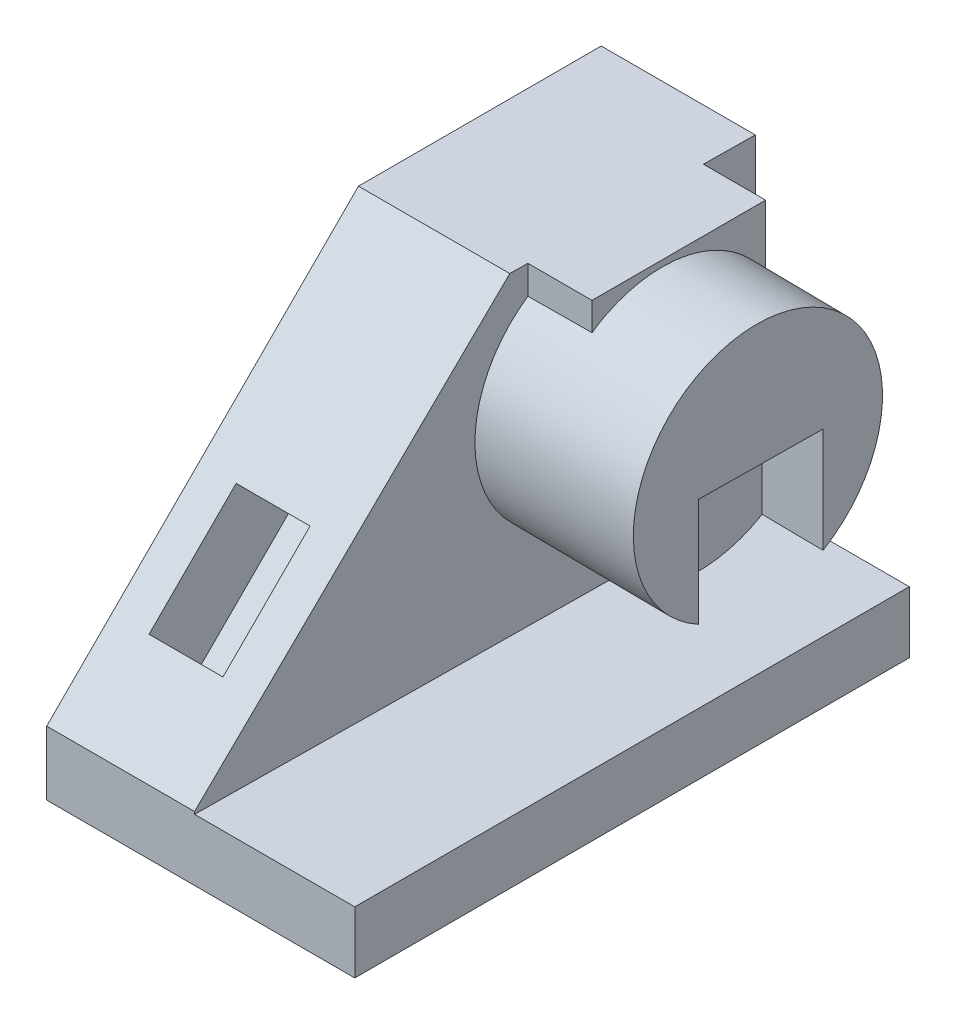
ISO-10303-21;
HEADER;
FILE_DESCRIPTION(('STEP AP214'),'2;1');
FILE_NAME('part.step','',(''),(''),'','','');
FILE_SCHEMA(('AUTOMOTIVE_DESIGN { 1 0 10303 214 1 1 1 1 }'));
ENDSEC;
DATA;
#1=APPLICATION_CONTEXT('core data for automotive mechanical design processes');
#2=APPLICATION_PROTOCOL_DEFINITION('international standard','automotive_design',2000,#1);
#3=PRODUCT_CONTEXT('',#1,'mechanical');
#4=PRODUCT('Part','Part','',(#3));
#5=PRODUCT_RELATED_PRODUCT_CATEGORY('part','',(#4));
#6=PRODUCT_DEFINITION_FORMATION('','',#4);
#7=PRODUCT_DEFINITION_CONTEXT('part definition',#1,'design');
#8=PRODUCT_DEFINITION('design','',#6,#7);
#9=PRODUCT_DEFINITION_SHAPE('','',#8);
#10=(LENGTH_UNIT() NAMED_UNIT(*) SI_UNIT(.MILLI.,.METRE.));
#11=(NAMED_UNIT(*) PLANE_ANGLE_UNIT() SI_UNIT($,.RADIAN.));
#12=(NAMED_UNIT(*) SI_UNIT($,.STERADIAN.) SOLID_ANGLE_UNIT());
#13=UNCERTAINTY_MEASURE_WITH_UNIT(LENGTH_MEASURE(1.E-05),#10,'distance_accuracy_value','');
#14=(GEOMETRIC_REPRESENTATION_CONTEXT(3) GLOBAL_UNCERTAINTY_ASSIGNED_CONTEXT((#13)) GLOBAL_UNIT_ASSIGNED_CONTEXT((#10,
#11,#12)) REPRESENTATION_CONTEXT('',''));
#15=CARTESIAN_POINT('',(0.,0.,0.));
#16=DIRECTION('',(0.,0.,1.));
#17=DIRECTION('',(1.,0.,0.));
#18=AXIS2_PLACEMENT_3D('',#15,#16,#17);
#19=CARTESIAN_POINT('',(-15.4419889502762,10.,45.));
#20=DIRECTION('',(1.,0.,0.));
#21=DIRECTION('',(0.,0.,-1.));
#22=AXIS2_PLACEMENT_3D('',#19,#20,#21);
#23=PLANE('',#22);
#24=DIRECTION('',(0.,-1.,0.));
#25=VECTOR('',#24,1.);
#26=CARTESIAN_POINT('',(-15.4419889502762,10.,45.));
#27=LINE('',#26,#25);
#28=CARTESIAN_POINT('',(-15.4419889502763,10.4020202535532,45.));
#29=VERTEX_POINT('',#28);
#30=CARTESIAN_POINT('',(-15.4419889502762,0.,45.));
#31=VERTEX_POINT('',#30);
#32=EDGE_CURVE('E303',#29,#31,#27,.T.);
#33=ORIENTED_EDGE('',*,*,#32,.F.);
#34=DIRECTION('',(0.,-0.707106781186549,0.707106781186546));
#35=VECTOR('',#34,1.);
#36=CARTESIAN_POINT('',(-15.4419889502763,-28.4088608780224,83.8108811315755));
#37=LINE('',#36,#35);
#38=CARTESIAN_POINT('',(-15.4419889502762,61.,-5.59797974644655));
#39=VERTEX_POINT('',#38);
#40=EDGE_CURVE('E203',#39,#29,#37,.T.);
#41=ORIENTED_EDGE('',*,*,#40,.F.);
#42=DIRECTION('',(0.,0.,1.));
#43=VECTOR('',#42,1.);
#44=CARTESIAN_POINT('',(-15.4419889502763,61.,-45.));
#45=LINE('',#44,#43);
#46=CARTESIAN_POINT('',(-15.4419889502763,61.,-45.));
#47=VERTEX_POINT('',#46);
#48=EDGE_CURVE('E220',#47,#39,#45,.T.);
#49=ORIENTED_EDGE('',*,*,#48,.F.);
#50=DIRECTION('',(0.,-1.,0.));
#51=VECTOR('',#50,1.);
#52=CARTESIAN_POINT('',(-15.4419889502762,10.,-45.));
#53=LINE('',#52,#51);
#54=CARTESIAN_POINT('',(-15.4419889502762,0.,-45.));
#55=VERTEX_POINT('',#54);
#56=EDGE_CURVE('E290',#47,#55,#53,.T.);
#57=ORIENTED_EDGE('',*,*,#56,.T.);
#58=DIRECTION('',(0.,0.,1.));
#59=VECTOR('',#58,1.);
#60=CARTESIAN_POINT('',(-15.4419889502762,0.,45.));
#61=LINE('',#60,#59);
#62=EDGE_CURVE('E280',#55,#31,#61,.T.);
#63=ORIENTED_EDGE('',*,*,#62,.T.);
#64=EDGE_LOOP('',(#33,#41,#49,#57,#63));
#65=FACE_BOUND('',#64,.T.);
#66=ADVANCED_FACE('F41',(#65),#23,.F.);
#67=CARTESIAN_POINT('',(34.5580110497238,10.,45.));
#68=DIRECTION('',(0.,0.,-1.));
#69=DIRECTION('',(-1.,0.,0.));
#70=AXIS2_PLACEMENT_3D('',#67,#68,#69);
#71=PLANE('',#70);
#72=DIRECTION('',(0.,-1.,0.));
#73=VECTOR('',#72,1.);
#74=CARTESIAN_POINT('',(8.55801104972375,60.,45.));
#75=LINE('',#74,#73);
#76=CARTESIAN_POINT('',(8.55801104972375,10.4020202535532,45.));
#77=VERTEX_POINT('',#76);
#78=CARTESIAN_POINT('',(8.55801104972376,10.,45.));
#79=VERTEX_POINT('',#78);
#80=EDGE_CURVE('E279',#77,#79,#75,.T.);
#81=ORIENTED_EDGE('',*,*,#80,.F.);
#82=DIRECTION('',(-1.,0.,0.));
#83=VECTOR('',#82,1.);
#84=CARTESIAN_POINT('',(34.5580110497238,10.4020202535532,45.));
#85=LINE('',#84,#83);
#86=EDGE_CURVE('E214',#77,#29,#85,.T.);
#87=ORIENTED_EDGE('',*,*,#86,.T.);
#88=ORIENTED_EDGE('',*,*,#32,.T.);
#89=DIRECTION('',(1.,0.,0.));
#90=VECTOR('',#89,1.);
#91=CARTESIAN_POINT('',(34.5580110497238,0.,45.));
#92=LINE('',#91,#90);
#93=CARTESIAN_POINT('',(34.5580110497238,0.,45.));
#94=VERTEX_POINT('',#93);
#95=EDGE_CURVE('E288',#31,#94,#92,.T.);
#96=ORIENTED_EDGE('',*,*,#95,.T.);
#97=DIRECTION('',(0.,-1.,0.));
#98=VECTOR('',#97,1.);
#99=CARTESIAN_POINT('',(34.5580110497238,10.,45.));
#100=LINE('',#99,#98);
#101=CARTESIAN_POINT('',(34.5580110497238,10.,45.));
#102=VERTEX_POINT('',#101);
#103=EDGE_CURVE('E297',#102,#94,#100,.T.);
#104=ORIENTED_EDGE('',*,*,#103,.F.);
#105=DIRECTION('',(1.,0.,0.));
#106=VECTOR('',#105,1.);
#107=CARTESIAN_POINT('',(34.5580110497238,10.,45.));
#108=LINE('',#107,#106);
#109=EDGE_CURVE('E278',#79,#102,#108,.T.);
#110=ORIENTED_EDGE('',*,*,#109,.F.);
#111=EDGE_LOOP('',(#81,#87,#88,#96,#104,#110));
#112=FACE_BOUND('',#111,.T.);
#113=ADVANCED_FACE('F360',(#112),#71,.F.);
#114=CARTESIAN_POINT('',(34.5580110497238,10.,45.));
#115=DIRECTION('',(-1.,0.,0.));
#116=DIRECTION('',(0.,0.,1.));
#117=AXIS2_PLACEMENT_3D('',#114,#115,#116);
#118=PLANE('',#117);
#119=DIRECTION('',(0.,0.,-1.));
#120=VECTOR('',#119,1.);
#121=CARTESIAN_POINT('',(34.5580110497238,0.,45.));
#122=LINE('',#121,#120);
#123=CARTESIAN_POINT('',(34.5580110497238,0.,-45.));
#124=VERTEX_POINT('',#123);
#125=EDGE_CURVE('E292',#94,#124,#122,.T.);
#126=ORIENTED_EDGE('',*,*,#125,.T.);
#127=DIRECTION('',(0.,-1.,0.));
#128=VECTOR('',#127,1.);
#129=CARTESIAN_POINT('',(34.5580110497238,10.,-45.));
#130=LINE('',#129,#128);
#131=CARTESIAN_POINT('',(34.5580110497238,10.,-45.));
#132=VERTEX_POINT('',#131);
#133=EDGE_CURVE('E300',#132,#124,#130,.T.);
#134=ORIENTED_EDGE('',*,*,#133,.F.);
#135=DIRECTION('',(0.,0.,-1.));
#136=VECTOR('',#135,1.);
#137=CARTESIAN_POINT('',(34.5580110497238,10.,45.));
#138=LINE('',#137,#136);
#139=EDGE_CURVE('E281',#102,#132,#138,.T.);
#140=ORIENTED_EDGE('',*,*,#139,.F.);
#141=ORIENTED_EDGE('',*,*,#103,.T.);
#142=EDGE_LOOP('',(#126,#134,#140,#141));
#143=FACE_BOUND('',#142,.T.);
#144=ADVANCED_FACE('F361',(#143),#118,.F.);
#145=CARTESIAN_POINT('',(34.5580110497238,10.,-45.));
#146=DIRECTION('',(0.,0.,1.));
#147=DIRECTION('',(1.,0.,0.));
#148=AXIS2_PLACEMENT_3D('',#145,#146,#147);
#149=PLANE('',#148);
#150=DIRECTION('',(0.,-1.,0.));
#151=VECTOR('',#150,1.);
#152=CARTESIAN_POINT('',(9.55801104972376,60.,-45.));
#153=LINE('',#152,#151);
#154=CARTESIAN_POINT('',(9.55801104972376,61.,-45.));
#155=VERTEX_POINT('',#154);
#156=CARTESIAN_POINT('',(9.55801104972376,10.,-45.));
#157=VERTEX_POINT('',#156);
#158=EDGE_CURVE('E274',#155,#157,#153,.T.);
#159=ORIENTED_EDGE('',*,*,#158,.T.);
#160=DIRECTION('',(-1.,0.,0.));
#161=VECTOR('',#160,1.);
#162=CARTESIAN_POINT('',(34.5580110497238,10.,-45.));
#163=LINE('',#162,#161);
#164=EDGE_CURVE('E282',#132,#157,#163,.T.);
#165=ORIENTED_EDGE('',*,*,#164,.F.);
#166=ORIENTED_EDGE('',*,*,#133,.T.);
#167=DIRECTION('',(-1.,0.,0.));
#168=VECTOR('',#167,1.);
#169=CARTESIAN_POINT('',(34.5580110497238,0.,-45.));
#170=LINE('',#169,#168);
#171=EDGE_CURVE('E285',#124,#55,#170,.T.);
#172=ORIENTED_EDGE('',*,*,#171,.T.);
#173=ORIENTED_EDGE('',*,*,#56,.F.);
#174=DIRECTION('',(-1.,0.,0.));
#175=VECTOR('',#174,1.);
#176=CARTESIAN_POINT('',(9.55801104972376,61.,-45.));
#177=LINE('',#176,#175);
#178=EDGE_CURVE('E213',#155,#47,#177,.T.);
#179=ORIENTED_EDGE('',*,*,#178,.F.);
#180=EDGE_LOOP('',(#159,#165,#166,#172,#173,#179));
#181=FACE_BOUND('',#180,.T.);
#182=ADVANCED_FACE('F331',(#181),#149,.F.);
#183=CARTESIAN_POINT('',(0.,10.,0.));
#184=DIRECTION('',(0.,1.,0.));
#185=DIRECTION('',(0.,0.,1.));
#186=AXIS2_PLACEMENT_3D('',#183,#184,#185);
#187=PLANE('',#186);
#188=DIRECTION('',(0.011110425303555,0.,-0.999938277319943));
#189=VECTOR('',#188,1.);
#190=CARTESIAN_POINT('',(8.55801104972375,10.,45.));
#191=LINE('',#190,#189);
#192=EDGE_CURVE('E268',#79,#157,#191,.T.);
#193=ORIENTED_EDGE('',*,*,#192,.F.);
#194=ORIENTED_EDGE('',*,*,#109,.T.);
#195=ORIENTED_EDGE('',*,*,#139,.T.);
#196=ORIENTED_EDGE('',*,*,#164,.T.);
#197=EDGE_LOOP('',(#193,#194,#195,#196));
#198=FACE_BOUND('',#197,.T.);
#199=ADVANCED_FACE('F372',(#198),#187,.T.);
#200=CARTESIAN_POINT('',(0.,0.,0.));
#201=DIRECTION('',(0.,1.,0.));
#202=DIRECTION('',(0.,0.,1.));
#203=AXIS2_PLACEMENT_3D('',#200,#201,#202);
#204=PLANE('',#203);
#205=ORIENTED_EDGE('',*,*,#62,.F.);
#206=ORIENTED_EDGE('',*,*,#171,.F.);
#207=ORIENTED_EDGE('',*,*,#125,.F.);
#208=ORIENTED_EDGE('',*,*,#95,.F.);
#209=EDGE_LOOP('',(#205,#206,#207,#208));
#210=FACE_BOUND('',#209,.T.);
#211=ADVANCED_FACE('F374',(#210),#204,.F.);
#212=CARTESIAN_POINT('',(8.55801104972375,60.,45.));
#213=DIRECTION('',(-0.999938277319942,0.,-0.011110425303555));
#214=DIRECTION('',(-0.011110425303555,0.,0.999938277319942));
#215=AXIS2_PLACEMENT_3D('',#212,#213,#214);
#216=PLANE('',#215);
#217=DIRECTION('',(0.0111104253035549,0.,-0.999938277319942));
#218=VECTOR('',#217,1.);
#219=CARTESIAN_POINT('',(9.0024554941682,61.,5.));
#220=LINE('',#219,#218);
#221=CARTESIAN_POINT('',(9.12021082468428,61.,-5.59797974644659));
#222=VERTEX_POINT('',#221);
#223=CARTESIAN_POINT('',(9.15254596288799,61.,-8.50814218478106));
#224=VERTEX_POINT('',#223);
#225=EDGE_CURVE('E219',#222,#224,#220,.T.);
#226=ORIENTED_EDGE('',*,*,#225,.F.);
#227=DIRECTION('',(-0.00785649953237235,-0.70708495791351,0.707084957913508));
#228=VECTOR('',#227,1.);
#229=CARTESIAN_POINT('',(8.83353837378895,35.1994794194208,20.2025408341325));
#230=LINE('',#229,#228);
#231=EDGE_CURVE('E61',#222,#77,#230,.T.);
#232=ORIENTED_EDGE('',*,*,#231,.T.);
#233=ORIENTED_EDGE('',*,*,#80,.T.);
#234=ORIENTED_EDGE('',*,*,#192,.T.);
#235=ORIENTED_EDGE('',*,*,#158,.F.);
#236=DIRECTION('',(0.0111104253035545,0.,-0.999938277319942));
#237=VECTOR('',#236,1.);
#238=CARTESIAN_POINT('',(9.46553831809246,61.,-36.6774541531825));
#239=LINE('',#238,#237);
#240=CARTESIAN_POINT('',(9.46553831809246,61.,-36.6774541531825));
#241=VERTEX_POINT('',#240);
#242=EDGE_CURVE('E233',#241,#155,#239,.T.);
#243=ORIENTED_EDGE('',*,*,#242,.F.);
#244=DIRECTION('',(0.,1.,0.));
#245=VECTOR('',#244,1.);
#246=CARTESIAN_POINT('',(9.46553831809246,40.,-36.6774541531825));
#247=LINE('',#246,#245);
#248=CARTESIAN_POINT('',(9.46553831809246,51.039912039484,-36.6774541531825));
#249=VERTEX_POINT('',#248);
#250=EDGE_CURVE('E232',#249,#241,#247,.T.);
#251=ORIENTED_EDGE('',*,*,#250,.F.);
#252=CARTESIAN_POINT('',(9.28025041713489,40.,-20.0015430670015));
#253=DIRECTION('',(0.999938277319943,0.,0.011110425303555));
#254=DIRECTION('',(0.011110425303555,0.,-0.999938277319943));
#255=AXIS2_PLACEMENT_3D('',#252,#253,#254);
#256=CIRCLE('',#255,20.);
#257=CARTESIAN_POINT('',(9.15254596288799,56.3672058621177,-8.50814218478106));
#258=VERTEX_POINT('',#257);
#259=EDGE_CURVE('E267',#258,#249,#256,.T.);
#260=ORIENTED_EDGE('',*,*,#259,.F.);
#261=DIRECTION('',(0.,1.,0.));
#262=VECTOR('',#261,1.);
#263=CARTESIAN_POINT('',(9.15254596288799,40.,-8.50814218478106));
#264=LINE('',#263,#262);
#265=EDGE_CURVE('E234',#258,#224,#264,.T.);
#266=ORIENTED_EDGE('',*,*,#265,.T.);
#267=EDGE_LOOP('',(#226,#232,#233,#234,#235,#243,#251,#260,#266));
#268=FACE_BOUND('',#267,.T.);
#269=ADVANCED_FACE('F328',(#268),#216,.F.);
#270=CARTESIAN_POINT('',(35.2786456274534,40.,-19.712672009109));
#271=DIRECTION('',(-0.999938277319943,0.,-0.011110425303555));
#272=DIRECTION('',(-0.011110425303555,0.,0.999938277319943));
#273=AXIS2_PLACEMENT_3D('',#270,#271,#272);
#274=CYLINDRICAL_SURFACE('',#273,20.);
#275=CARTESIAN_POINT('',(35.2786456274534,40.,-19.712672009109));
#276=DIRECTION('',(0.999938277319943,0.,0.011110425303555));
#277=DIRECTION('',(0.011110425303555,0.,-0.999938277319943));
#278=AXIS2_PLACEMENT_3D('',#275,#276,#277);
#279=CIRCLE('',#278,20.);
#280=CARTESIAN_POINT('',(35.3948087110377,22.9504773076578,-30.1673495316977));
#281=VERTEX_POINT('',#280);
#282=CARTESIAN_POINT('',(35.1726002049666,22.4244733176461,-10.1685839852988));
#283=VERTEX_POINT('',#282);
#284=EDGE_CURVE('E270',#281,#283,#279,.T.);
#285=ORIENTED_EDGE('',*,*,#284,.F.);
#286=DIRECTION('',(-0.999938277319943,0.,-0.011110425303555));
#287=VECTOR('',#286,1.);
#288=CARTESIAN_POINT('',(35.3948087110377,22.9504773076578,-30.1673495316977));
#289=LINE('',#288,#287);
#290=CARTESIAN_POINT('',(25.3954259378383,22.9504773076578,-30.2784537847332));
#291=VERTEX_POINT('',#290);
#292=EDGE_CURVE('E263',#281,#291,#289,.T.);
#293=ORIENTED_EDGE('',*,*,#292,.T.);
#294=CARTESIAN_POINT('',(25.279262854254,40.,-19.8237762621446));
#295=DIRECTION('',(0.999938277319943,0.,0.011110425303555));
#296=DIRECTION('',(0.011110425303555,0.,-0.999938277319943));
#297=AXIS2_PLACEMENT_3D('',#294,#295,#296);
#298=CIRCLE('',#297,20.);
#299=CARTESIAN_POINT('',(25.1732174317672,22.4244733176461,-10.2796882383344));
#300=VERTEX_POINT('',#299);
#301=EDGE_CURVE('E308',#300,#291,#298,.T.);
#302=ORIENTED_EDGE('',*,*,#301,.F.);
#303=DIRECTION('',(-0.999938277319943,0.,-0.011110425303555));
#304=VECTOR('',#303,1.);
#305=CARTESIAN_POINT('',(35.1726002049666,22.4244733176461,-10.1685839852988));
#306=LINE('',#305,#304);
#307=EDGE_CURVE('E258',#300,#283,#306,.F.);
#308=ORIENTED_EDGE('',*,*,#307,.T.);
#309=EDGE_LOOP('',(#285,#293,#302,#308));
#310=FACE_BOUND('',#309,.T.);
#311=ORIENTED_EDGE('',*,*,#259,.T.);
#312=CARTESIAN_POINT('',(-1491.55174733915,40.,-36.6774541531825));
#313=DIRECTION('',(0.,0.,-1.));
#314=DIRECTION('',(-1.,0.,0.));
#315=AXIS2_PLACEMENT_3D('',#312,#313,#314);
#316=ELLIPSE('',#315,1800.11110768196,20.);
#317=CARTESIAN_POINT('',(19.5580110497238,50.8686272432883,-36.6774541531825));
#318=VERTEX_POINT('',#317);
#319=EDGE_CURVE('E48',#249,#318,#316,.T.);
#320=ORIENTED_EDGE('',*,*,#319,.T.);
#321=CARTESIAN_POINT('',(19.5580110497238,40.,-19.8873457266394));
#322=DIRECTION('',(1.,0.,0.));
#323=DIRECTION('',(0.,0.,-1.));
#324=AXIS2_PLACEMENT_3D('',#321,#322,#323);
#325=ELLIPSE('',#324,20.0012345297996,20.);
#326=CARTESIAN_POINT('',(19.5580110497238,56.4477874116639,-8.50814218478106));
#327=VERTEX_POINT('',#326);
#328=EDGE_CURVE('E312',#318,#327,#325,.T.);
#329=ORIENTED_EDGE('',*,*,#328,.T.);
#330=CARTESIAN_POINT('',(1043.68632981697,40.,-8.50814218478106));
#331=DIRECTION('',(0.,0.,1.));
#332=DIRECTION('',(-1.,0.,0.));
#333=AXIS2_PLACEMENT_3D('',#330,#331,#332);
#334=ELLIPSE('',#333,1800.11110768196,20.);
#335=EDGE_CURVE('E309',#327,#258,#334,.T.);
#336=ORIENTED_EDGE('',*,*,#335,.T.);
#337=EDGE_LOOP('',(#311,#320,#329,#336));
#338=FACE_BOUND('',#337,.T.);
#339=ADVANCED_FACE('F319',(#310,#338),#274,.T.);
#340=CARTESIAN_POINT('',(35.2786456274534,40.,-19.712672009109));
#341=DIRECTION('',(0.999938277319943,0.,0.011110425303555));
#342=DIRECTION('',(0.011110425303555,0.,-0.999938277319943));
#343=AXIS2_PLACEMENT_3D('',#340,#341,#342);
#344=PLANE('',#343);
#345=DIRECTION('',(0.,1.,0.));
#346=VECTOR('',#345,1.);
#347=CARTESIAN_POINT('',(35.3948087110377,40.,-30.1673495316977));
#348=LINE('',#347,#346);
#349=CARTESIAN_POINT('',(35.3948087110377,40.,-30.1673495316988));
#350=VERTEX_POINT('',#349);
#351=EDGE_CURVE('E304',#281,#350,#348,.T.);
#352=ORIENTED_EDGE('',*,*,#351,.F.);
#353=ORIENTED_EDGE('',*,*,#284,.T.);
#354=DIRECTION('',(0.,-1.,0.));
#355=VECTOR('',#354,1.);
#356=CARTESIAN_POINT('',(35.1726002049666,40.,-10.1685839852988));
#357=LINE('',#356,#355);
#358=CARTESIAN_POINT('',(35.1726002049666,40.,-10.1685839852988));
#359=VERTEX_POINT('',#358);
#360=EDGE_CURVE('E250',#359,#283,#357,.T.);
#361=ORIENTED_EDGE('',*,*,#360,.F.);
#362=DIRECTION('',(-0.0111104253035552,0.,0.999938277319943));
#363=VECTOR('',#362,1.);
#364=CARTESIAN_POINT('',(35.1726002049666,40.,-10.1685839852988));
#365=LINE('',#364,#363);
#366=EDGE_CURVE('E240',#350,#359,#365,.T.);
#367=ORIENTED_EDGE('',*,*,#366,.F.);
#368=EDGE_LOOP('',(#352,#353,#361,#367));
#369=FACE_BOUND('',#368,.T.);
#370=ADVANCED_FACE('F383',(#369),#344,.T.);
#371=CARTESIAN_POINT('',(25.2843216848027,40.,-20.2790710115338));
#372=DIRECTION('',(0.999938277319943,0.,0.011110425303555));
#373=DIRECTION('',(0.011110425303555,0.,-0.999938277319943));
#374=AXIS2_PLACEMENT_3D('',#371,#372,#373);
#375=PLANE('',#374);
#376=ORIENTED_EDGE('',*,*,#301,.T.);
#377=DIRECTION('',(0.,1.,0.));
#378=VECTOR('',#377,1.);
#379=CARTESIAN_POINT('',(25.3954259378383,40.,-30.2784537847332));
#380=LINE('',#379,#378);
#381=CARTESIAN_POINT('',(25.3954259378383,40.,-30.2784537847332));
#382=VERTEX_POINT('',#381);
#383=EDGE_CURVE('E242',#291,#382,#380,.T.);
#384=ORIENTED_EDGE('',*,*,#383,.T.);
#385=DIRECTION('',(-0.0111104253035552,0.,0.999938277319943));
#386=VECTOR('',#385,1.);
#387=CARTESIAN_POINT('',(25.1732174317672,40.,-10.2796882383344));
#388=LINE('',#387,#386);
#389=CARTESIAN_POINT('',(25.1732174317672,40.,-10.2796882383344));
#390=VERTEX_POINT('',#389);
#391=EDGE_CURVE('E246',#382,#390,#388,.T.);
#392=ORIENTED_EDGE('',*,*,#391,.T.);
#393=DIRECTION('',(0.,-1.,0.));
#394=VECTOR('',#393,1.);
#395=CARTESIAN_POINT('',(25.1732174317672,40.,-10.2796882383344));
#396=LINE('',#395,#394);
#397=EDGE_CURVE('E249',#390,#300,#396,.T.);
#398=ORIENTED_EDGE('',*,*,#397,.T.);
#399=EDGE_LOOP('',(#376,#384,#392,#398));
#400=FACE_BOUND('',#399,.T.);
#401=ADVANCED_FACE('F388',(#400),#375,.T.);
#402=CARTESIAN_POINT('',(25.3954259378383,40.,-30.2784537847332));
#403=DIRECTION('',(0.011110425303555,0.,-0.999938277319943));
#404=DIRECTION('',(-0.999938277319943,0.,-0.011110425303555));
#405=AXIS2_PLACEMENT_3D('',#402,#403,#404);
#406=PLANE('',#405);
#407=ORIENTED_EDGE('',*,*,#351,.T.);
#408=DIRECTION('',(0.999938277319943,0.,0.011110425303555));
#409=VECTOR('',#408,1.);
#410=CARTESIAN_POINT('',(25.3954259378383,40.,-30.2784537847332));
#411=LINE('',#410,#409);
#412=EDGE_CURVE('E254',#382,#350,#411,.T.);
#413=ORIENTED_EDGE('',*,*,#412,.F.);
#414=ORIENTED_EDGE('',*,*,#383,.F.);
#415=ORIENTED_EDGE('',*,*,#292,.F.);
#416=EDGE_LOOP('',(#407,#413,#414,#415));
#417=FACE_BOUND('',#416,.T.);
#418=ADVANCED_FACE('F391',(#417),#406,.F.);
#419=CARTESIAN_POINT('',(25.1732174317672,40.,-10.2796882383344));
#420=DIRECTION('',(-0.011110425303555,0.,0.999938277319943));
#421=DIRECTION('',(0.999938277319943,0.,0.011110425303555));
#422=AXIS2_PLACEMENT_3D('',#419,#420,#421);
#423=PLANE('',#422);
#424=ORIENTED_EDGE('',*,*,#397,.F.);
#425=DIRECTION('',(0.999938277319943,0.,0.011110425303555));
#426=VECTOR('',#425,1.);
#427=CARTESIAN_POINT('',(25.1732174317672,40.,-10.2796882383344));
#428=LINE('',#427,#426);
#429=EDGE_CURVE('E256',#390,#359,#428,.T.);
#430=ORIENTED_EDGE('',*,*,#429,.T.);
#431=ORIENTED_EDGE('',*,*,#360,.T.);
#432=ORIENTED_EDGE('',*,*,#307,.F.);
#433=EDGE_LOOP('',(#424,#430,#431,#432));
#434=FACE_BOUND('',#433,.T.);
#435=ADVANCED_FACE('F392',(#434),#423,.F.);
#436=CARTESIAN_POINT('',(25.1732174317672,40.,-10.2796882383344));
#437=DIRECTION('',(0.,1.,0.));
#438=DIRECTION('',(0.,0.,1.));
#439=AXIS2_PLACEMENT_3D('',#436,#437,#438);
#440=PLANE('',#439);
#441=ORIENTED_EDGE('',*,*,#366,.T.);
#442=ORIENTED_EDGE('',*,*,#429,.F.);
#443=ORIENTED_EDGE('',*,*,#391,.F.);
#444=ORIENTED_EDGE('',*,*,#412,.T.);
#445=EDGE_LOOP('',(#441,#442,#443,#444));
#446=FACE_BOUND('',#445,.T.);
#447=ADVANCED_FACE('F358',(#446),#440,.F.);
#448=CARTESIAN_POINT('',(19.5580110497238,40.,-36.6774541531825));
#449=DIRECTION('',(0.,0.,-1.));
#450=DIRECTION('',(-1.,0.,0.));
#451=AXIS2_PLACEMENT_3D('',#448,#449,#450);
#452=PLANE('',#451);
#453=ORIENTED_EDGE('',*,*,#319,.F.);
#454=ORIENTED_EDGE('',*,*,#250,.T.);
#455=DIRECTION('',(-1.,0.,0.));
#456=VECTOR('',#455,1.);
#457=CARTESIAN_POINT('',(19.5580110497238,61.,-36.6774541531825));
#458=LINE('',#457,#456);
#459=CARTESIAN_POINT('',(19.5580110497238,61.,-36.6774541531825));
#460=VERTEX_POINT('',#459);
#461=EDGE_CURVE('E226',#460,#241,#458,.T.);
#462=ORIENTED_EDGE('',*,*,#461,.F.);
#463=DIRECTION('',(0.,1.,0.));
#464=VECTOR('',#463,1.);
#465=CARTESIAN_POINT('',(19.5580110497238,40.,-36.6774541531825));
#466=LINE('',#465,#464);
#467=EDGE_CURVE('E238',#318,#460,#466,.T.);
#468=ORIENTED_EDGE('',*,*,#467,.F.);
#469=EDGE_LOOP('',(#453,#454,#462,#468));
#470=FACE_BOUND('',#469,.T.);
#471=ADVANCED_FACE('F325',(#470),#452,.T.);
#472=CARTESIAN_POINT('',(19.5580110497238,40.,-8.50814218478106));
#473=DIRECTION('',(1.,0.,0.));
#474=DIRECTION('',(0.,0.,-1.));
#475=AXIS2_PLACEMENT_3D('',#472,#473,#474);
#476=PLANE('',#475);
#477=ORIENTED_EDGE('',*,*,#328,.F.);
#478=ORIENTED_EDGE('',*,*,#467,.T.);
#479=DIRECTION('',(0.,0.,-1.));
#480=VECTOR('',#479,1.);
#481=CARTESIAN_POINT('',(19.5580110497238,61.,-8.50814218478106));
#482=LINE('',#481,#480);
#483=CARTESIAN_POINT('',(19.5580110497238,61.,-8.50814218478106));
#484=VERTEX_POINT('',#483);
#485=EDGE_CURVE('E223',#484,#460,#482,.T.);
#486=ORIENTED_EDGE('',*,*,#485,.F.);
#487=DIRECTION('',(0.,1.,0.));
#488=VECTOR('',#487,1.);
#489=CARTESIAN_POINT('',(19.5580110497238,40.,-8.50814218478106));
#490=LINE('',#489,#488);
#491=EDGE_CURVE('E239',#327,#484,#490,.T.);
#492=ORIENTED_EDGE('',*,*,#491,.F.);
#493=EDGE_LOOP('',(#477,#478,#486,#492));
#494=FACE_BOUND('',#493,.T.);
#495=ADVANCED_FACE('F348',(#494),#476,.T.);
#496=CARTESIAN_POINT('',(9.15254596288799,40.,-8.50814218478106));
#497=DIRECTION('',(0.,0.,1.));
#498=DIRECTION('',(1.,0.,0.));
#499=AXIS2_PLACEMENT_3D('',#496,#497,#498);
#500=PLANE('',#499);
#501=ORIENTED_EDGE('',*,*,#335,.F.);
#502=ORIENTED_EDGE('',*,*,#491,.T.);
#503=DIRECTION('',(1.,0.,0.));
#504=VECTOR('',#503,1.);
#505=CARTESIAN_POINT('',(9.15254596288799,61.,-8.50814218478106));
#506=LINE('',#505,#504);
#507=EDGE_CURVE('E225',#224,#484,#506,.T.);
#508=ORIENTED_EDGE('',*,*,#507,.F.);
#509=ORIENTED_EDGE('',*,*,#265,.F.);
#510=EDGE_LOOP('',(#501,#502,#508,#509));
#511=FACE_BOUND('',#510,.T.);
#512=ADVANCED_FACE('F343',(#511),#500,.T.);
#513=CARTESIAN_POINT('',(0.,61.,0.));
#514=DIRECTION('',(0.,1.,0.));
#515=DIRECTION('',(0.,0.,1.));
#516=AXIS2_PLACEMENT_3D('',#513,#514,#515);
#517=PLANE('',#516);
#518=DIRECTION('',(-1.,0.,0.));
#519=VECTOR('',#518,1.);
#520=CARTESIAN_POINT('',(0.,61.,-5.59797974644659));
#521=LINE('',#520,#519);
#522=EDGE_CURVE('E11',#222,#39,#521,.T.);
#523=ORIENTED_EDGE('',*,*,#522,.F.);
#524=ORIENTED_EDGE('',*,*,#225,.T.);
#525=ORIENTED_EDGE('',*,*,#507,.T.);
#526=ORIENTED_EDGE('',*,*,#485,.T.);
#527=ORIENTED_EDGE('',*,*,#461,.T.);
#528=ORIENTED_EDGE('',*,*,#242,.T.);
#529=ORIENTED_EDGE('',*,*,#178,.T.);
#530=ORIENTED_EDGE('',*,*,#48,.T.);
#531=EDGE_LOOP('',(#523,#524,#525,#526,#527,#528,#529,#530));
#532=FACE_BOUND('',#531,.T.);
#533=ADVANCED_FACE('F332',(#532),#517,.T.);
#534=CARTESIAN_POINT('',(0.,27.7010101267766,27.7010101267767));
#535=DIRECTION('',(0.,-0.707106781186546,-0.707106781186549));
#536=DIRECTION('',(0.,0.707106781186549,-0.707106781186546));
#537=AXIS2_PLACEMENT_3D('',#534,#535,#536);
#538=PLANE('',#537);
#539=DIRECTION('',(1.,0.,0.));
#540=VECTOR('',#539,1.);
#541=CARTESIAN_POINT('',(-9.44198895027625,21.0086219713515,34.3933982822018));
#542=LINE('',#541,#540);
#543=CARTESIAN_POINT('',(-9.44198895027625,21.0086219713515,34.3933982822018));
#544=VERTEX_POINT('',#543);
#545=CARTESIAN_POINT('',(2.55801104972375,21.0086219713515,34.3933982822018));
#546=VERTEX_POINT('',#545);
#547=EDGE_CURVE('E197',#544,#546,#542,.T.);
#548=ORIENTED_EDGE('',*,*,#547,.F.);
#549=DIRECTION('',(0.,-0.707106781186549,0.707106781186546));
#550=VECTOR('',#549,1.);
#551=CARTESIAN_POINT('',(-9.44198895027625,21.0086219713515,34.3933982822018));
#552=LINE('',#551,#550);
#553=CARTESIAN_POINT('',(-9.44198895027625,35.1507575950824,20.2512626584709));
#554=VERTEX_POINT('',#553);
#555=EDGE_CURVE('E54',#554,#544,#552,.T.);
#556=ORIENTED_EDGE('',*,*,#555,.F.);
#557=DIRECTION('',(-1.,0.,0.));
#558=VECTOR('',#557,1.);
#559=CARTESIAN_POINT('',(-9.44198895027625,35.1507575950824,20.2512626584709));
#560=LINE('',#559,#558);
#561=CARTESIAN_POINT('',(2.55801104972375,35.1507575950824,20.2512626584709));
#562=VERTEX_POINT('',#561);
#563=EDGE_CURVE('E188',#562,#554,#560,.T.);
#564=ORIENTED_EDGE('',*,*,#563,.F.);
#565=DIRECTION('',(0.,0.707106781186549,-0.707106781186546));
#566=VECTOR('',#565,1.);
#567=CARTESIAN_POINT('',(2.55801104972375,21.0086219713515,34.3933982822018));
#568=LINE('',#567,#566);
#569=EDGE_CURVE('E195',#546,#562,#568,.T.);
#570=ORIENTED_EDGE('',*,*,#569,.F.);
#571=EDGE_LOOP('',(#548,#556,#564,#570));
#572=FACE_BOUND('',#571,.T.);
#573=ORIENTED_EDGE('',*,*,#231,.F.);
#574=ORIENTED_EDGE('',*,*,#522,.T.);
#575=ORIENTED_EDGE('',*,*,#40,.T.);
#576=ORIENTED_EDGE('',*,*,#86,.F.);
#577=EDGE_LOOP('',(#573,#574,#575,#576));
#578=FACE_BOUND('',#577,.T.);
#579=ADVANCED_FACE('F471',(#572,#578),#538,.F.);
#580=CARTESIAN_POINT('',(-9.44198895027625,12.5233405971129,25.9081169079632));
#581=DIRECTION('',(-1.,0.,0.));
#582=DIRECTION('',(0.,0.,1.));
#583=AXIS2_PLACEMENT_3D('',#580,#581,#582);
#584=PLANE('',#583);
#585=ORIENTED_EDGE('',*,*,#555,.T.);
#586=DIRECTION('',(0.,0.707106781186546,0.707106781186549));
#587=VECTOR('',#586,1.);
#588=CARTESIAN_POINT('',(-9.44198895027625,12.5233405971129,25.9081169079632));
#589=LINE('',#588,#587);
#590=CARTESIAN_POINT('',(-9.44198895027625,12.5233405971129,25.9081169079632));
#591=VERTEX_POINT('',#590);
#592=EDGE_CURVE('E166',#591,#544,#589,.T.);
#593=ORIENTED_EDGE('',*,*,#592,.F.);
#594=DIRECTION('',(0.,-0.707106781186549,0.707106781186546));
#595=VECTOR('',#594,1.);
#596=CARTESIAN_POINT('',(-9.44198895027625,12.5233405971129,25.9081169079632));
#597=LINE('',#596,#595);
#598=CARTESIAN_POINT('',(-9.44198895027625,26.6654762208439,11.7659812842323));
#599=VERTEX_POINT('',#598);
#600=EDGE_CURVE('E175',#599,#591,#597,.T.);
#601=ORIENTED_EDGE('',*,*,#600,.F.);
#602=DIRECTION('',(0.,0.707106781186546,0.707106781186549));
#603=VECTOR('',#602,1.);
#604=CARTESIAN_POINT('',(-9.44198895027625,26.6654762208439,11.7659812842323));
#605=LINE('',#604,#603);
#606=EDGE_CURVE('E204',#599,#554,#605,.T.);
#607=ORIENTED_EDGE('',*,*,#606,.T.);
#608=EDGE_LOOP('',(#585,#593,#601,#607));
#609=FACE_BOUND('',#608,.T.);
#610=ADVANCED_FACE('F167',(#609),#584,.F.);
#611=CARTESIAN_POINT('',(-9.44198895027625,26.6654762208439,11.7659812842323));
#612=DIRECTION('',(0.,0.707106781186549,-0.707106781186546));
#613=DIRECTION('',(0.,0.707106781186546,0.707106781186549));
#614=AXIS2_PLACEMENT_3D('',#611,#612,#613);
#615=PLANE('',#614);
#616=ORIENTED_EDGE('',*,*,#563,.T.);
#617=ORIENTED_EDGE('',*,*,#606,.F.);
#618=DIRECTION('',(-1.,0.,0.));
#619=VECTOR('',#618,1.);
#620=CARTESIAN_POINT('',(-9.44198895027625,26.6654762208439,11.7659812842323));
#621=LINE('',#620,#619);
#622=CARTESIAN_POINT('',(2.55801104972375,26.6654762208439,11.7659812842323));
#623=VERTEX_POINT('',#622);
#624=EDGE_CURVE('E178',#623,#599,#621,.T.);
#625=ORIENTED_EDGE('',*,*,#624,.F.);
#626=DIRECTION('',(0.,0.707106781186546,0.707106781186549));
#627=VECTOR('',#626,1.);
#628=CARTESIAN_POINT('',(2.55801104972375,26.6654762208439,11.7659812842323));
#629=LINE('',#628,#627);
#630=EDGE_CURVE('E207',#623,#562,#629,.T.);
#631=ORIENTED_EDGE('',*,*,#630,.T.);
#632=EDGE_LOOP('',(#616,#617,#625,#631));
#633=FACE_BOUND('',#632,.T.);
#634=ADVANCED_FACE('F489',(#633),#615,.F.);
#635=CARTESIAN_POINT('',(2.55801104972375,12.5233405971129,25.9081169079632));
#636=DIRECTION('',(1.,0.,0.));
#637=DIRECTION('',(0.,0.,-1.));
#638=AXIS2_PLACEMENT_3D('',#635,#636,#637);
#639=PLANE('',#638);
#640=ORIENTED_EDGE('',*,*,#569,.T.);
#641=ORIENTED_EDGE('',*,*,#630,.F.);
#642=DIRECTION('',(0.,0.707106781186549,-0.707106781186546));
#643=VECTOR('',#642,1.);
#644=CARTESIAN_POINT('',(2.55801104972375,12.5233405971129,25.9081169079632));
#645=LINE('',#644,#643);
#646=CARTESIAN_POINT('',(2.55801104972375,12.5233405971129,25.9081169079632));
#647=VERTEX_POINT('',#646);
#648=EDGE_CURVE('E187',#647,#623,#645,.T.);
#649=ORIENTED_EDGE('',*,*,#648,.F.);
#650=DIRECTION('',(0.,0.707106781186546,0.707106781186549));
#651=VECTOR('',#650,1.);
#652=CARTESIAN_POINT('',(2.55801104972375,12.5233405971129,25.9081169079632));
#653=LINE('',#652,#651);
#654=EDGE_CURVE('E180',#647,#546,#653,.T.);
#655=ORIENTED_EDGE('',*,*,#654,.T.);
#656=EDGE_LOOP('',(#640,#641,#649,#655));
#657=FACE_BOUND('',#656,.T.);
#658=ADVANCED_FACE('F497',(#657),#639,.F.);
#659=CARTESIAN_POINT('',(-9.44198895027625,12.5233405971129,25.9081169079632));
#660=DIRECTION('',(0.,-0.707106781186549,0.707106781186546));
#661=DIRECTION('',(0.,-0.707106781186546,-0.707106781186549));
#662=AXIS2_PLACEMENT_3D('',#659,#660,#661);
#663=PLANE('',#662);
#664=ORIENTED_EDGE('',*,*,#547,.T.);
#665=ORIENTED_EDGE('',*,*,#654,.F.);
#666=DIRECTION('',(1.,0.,0.));
#667=VECTOR('',#666,1.);
#668=CARTESIAN_POINT('',(-9.44198895027625,12.5233405971129,25.9081169079632));
#669=LINE('',#668,#667);
#670=EDGE_CURVE('E181',#591,#647,#669,.T.);
#671=ORIENTED_EDGE('',*,*,#670,.F.);
#672=ORIENTED_EDGE('',*,*,#592,.T.);
#673=EDGE_LOOP('',(#664,#665,#671,#672));
#674=FACE_BOUND('',#673,.T.);
#675=ADVANCED_FACE('F185',(#674),#663,.F.);
#676=CARTESIAN_POINT('',(0.,19.215728752538,19.2157287525381));
#677=DIRECTION('',(0.,-0.707106781186546,-0.707106781186549));
#678=DIRECTION('',(0.,0.707106781186549,-0.707106781186546));
#679=AXIS2_PLACEMENT_3D('',#676,#677,#678);
#680=PLANE('',#679);
#681=ORIENTED_EDGE('',*,*,#600,.T.);
#682=ORIENTED_EDGE('',*,*,#670,.T.);
#683=ORIENTED_EDGE('',*,*,#648,.T.);
#684=ORIENTED_EDGE('',*,*,#624,.T.);
#685=EDGE_LOOP('',(#681,#682,#683,#684));
#686=FACE_BOUND('',#685,.T.);
#687=ADVANCED_FACE('F189',(#686),#680,.F.);
#688=CLOSED_SHELL('',(#66,#113,#144,#182,#199,#211,#269,#339,#370,#401,#418,#435,#447,#471,#495,
#512,#533,#579,#610,#634,#658,#675,#687));
#689=MANIFOLD_SOLID_BREP('B2',#688);
#690=ADVANCED_BREP_SHAPE_REPRESENTATION('',(#18,#689),#14);
#691=SHAPE_DEFINITION_REPRESENTATION(#9,#690);
ENDSEC;
END-ISO-10303-21;
